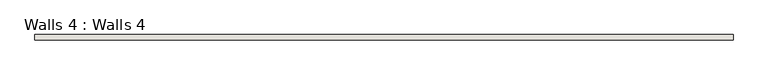
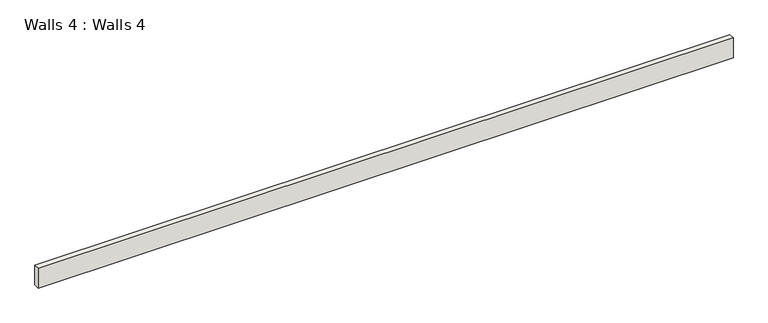
"""IFC4 building model written with IfcOpenShell, lengths in millimetres: wall geometry, Walls 4 : Walls 4."""

from ifc_helpers import new_model, si_unit, frame, origin, place, context, project, spatial, polyline, outline, extrude, source, transform, mapped, element, save


def walls_4_walls_4_28ce44a6(model_context):
    return source(origin(), model_context, "Body", "SweptSolid", [
        extrude(outline(polyline([(17663.6339443, -12649.0789019), (-18812.3660557, -12649.0789019), (-18812.3660557, -12367.9194855), (17663.6339443, -12367.9194855), (17663.6339443, -12649.0789019)])), frame((0.0, 0.0, 4570.0678272), z_axis=(0.0, 0.0, 1.0), x_axis=(1.0, 0.0, 0.0)), (0.0, 0.0, 1.0), 1100.5789247),
    ])


if __name__ == "__main__":
    model = new_model("IFC4")
    model_context = context("Model", 3, world=origin())
    ifc_project = project(units=[si_unit("LENGTHUNIT", "METRE", prefix="MILLI")], contexts=[model_context])
    site = spatial("IfcSite", under=ifc_project)
    building = spatial("IfcBuilding", under=site)
    placement = place(None, origin())
    walls_4_walls_4_shape = walls_4_walls_4_28ce44a6(model_context)
    element("IfcWall", 1, ObjectType="Walls 4 : Walls 4", at=placement, inside=building, context=model_context, shape_type="MappedRepresentation", body=[
        mapped(walls_4_walls_4_shape, transform((0.0, 0.0, 0.0), x_axis=(1.0, 0.0, 0.0), y_axis=(0.0, 1.0, 0.0), z_axis=(0.0, 0.0, 1.0))),
    ])
    save(model, "model.ifc")

# Revit data of these elements
# Element 1 (IfcWall, "Walls 4 : Walls 4")
#   Materials on its faces: "Default Wall"
# Materials
#   "Default Wall": colour RGB 80 80 80, transparency 0
